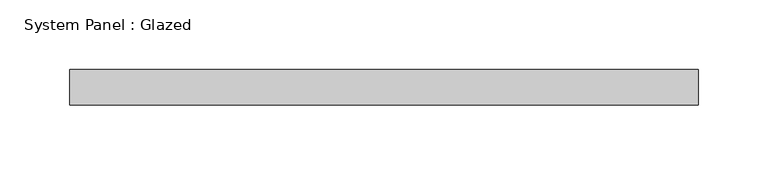
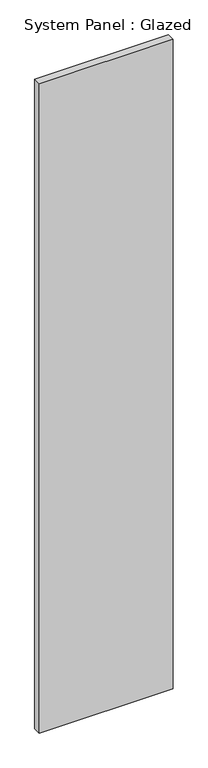
"""IFC4 building model written with IfcOpenShell, lengths in millimetres: plate geometry, System Panel : Glazed."""

from ifc_helpers import new_model, si_unit, origin, origin_with_axes, place, context, project, spatial, polyline, outline, extrude, source, transform, mapped, element, save


def system_panel_glazed_383feac9(model_context):
    return source(origin(), model_context, "Body", "SweptSolid", [
        extrude(outline(polyline([(225.4084635, 19.05), (-225.4084635, 19.05), (-225.4084635, 44.45), (225.4084635, 44.45), (225.4084635, 19.05)])), origin_with_axes(), (0.0, 0.0, 1.0), 2311.4),
    ])


if __name__ == "__main__":
    model = new_model("IFC4")
    model_context = context("Model", 3, world=origin())
    ifc_project = project(units=[si_unit("LENGTHUNIT", "METRE", prefix="MILLI")], contexts=[model_context])
    site = spatial("IfcSite", under=ifc_project)
    building = spatial("IfcBuilding", under=site)
    placement = place(None, origin())
    system_panel_glazed_shape = system_panel_glazed_383feac9(model_context)
    element("IfcPlate", 1, ObjectType="System Panel : Glazed", at=placement, inside=building, context=model_context, shape_type="MappedRepresentation", body=[
        mapped(system_panel_glazed_shape, transform((0.0, 0.0, 0.0), x_axis=(1.0, 0.0, 0.0), y_axis=(0.0, 1.0, 0.0), z_axis=(0.0, 0.0, 1.0))),
    ])
    save(model, "model.ifc")

# Revit data of these elements
# Type "System Panel : Glazed"
#   Construction Type Id = "GSP4R"
#   Analytic Construction = "1/8 in Pilkington single glazing"
#   Visual Light Transmittance = 0.9
#   Solar Heat Gain Coefficient = 0.86
#   Heat Transfer Coefficient (U) = 1.18115 BTU/(h·ft²·°F)
#   Define Thermal Properties by = 1
# Element 1 (IfcPlate, "System Panel : Glazed")
#   Materials on its faces: "Glass"
# Materials
#   "Glass": class "Glass", colour RGB 0 128 192, transparency 0.75, Description = "Soda Lime Glass", Cost = 0
